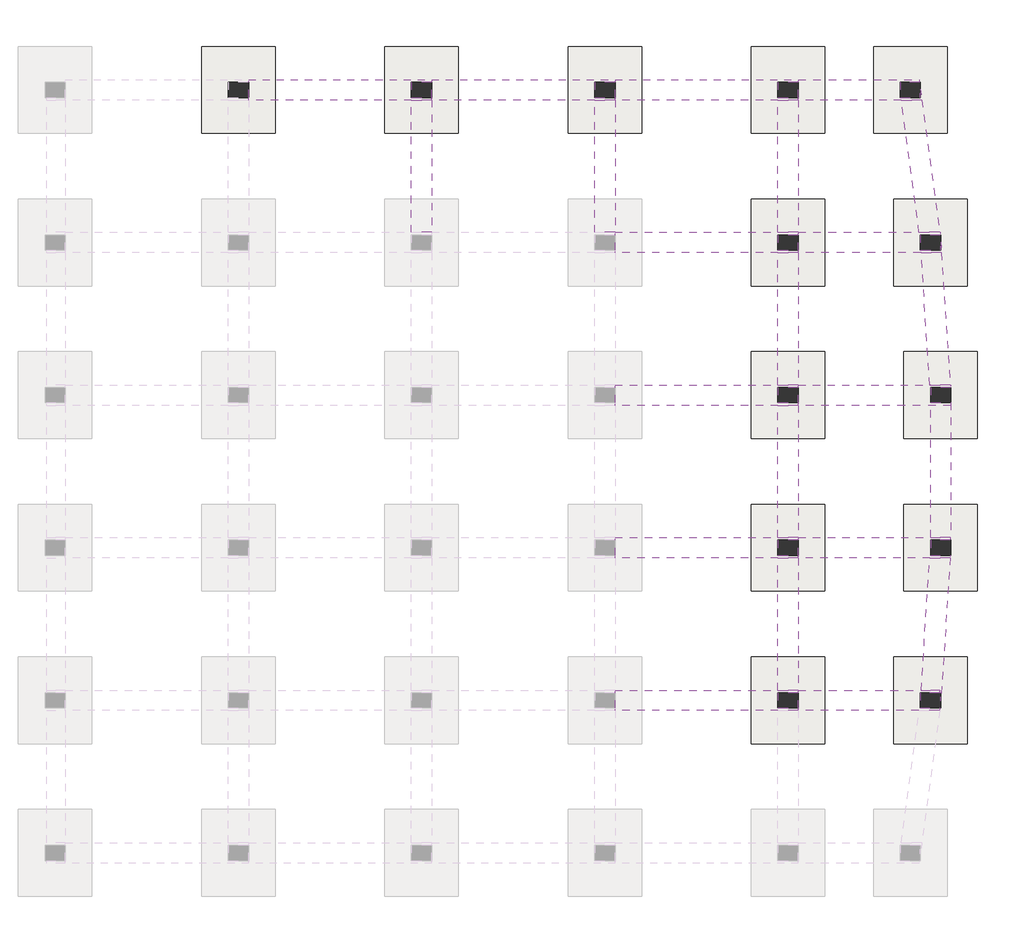
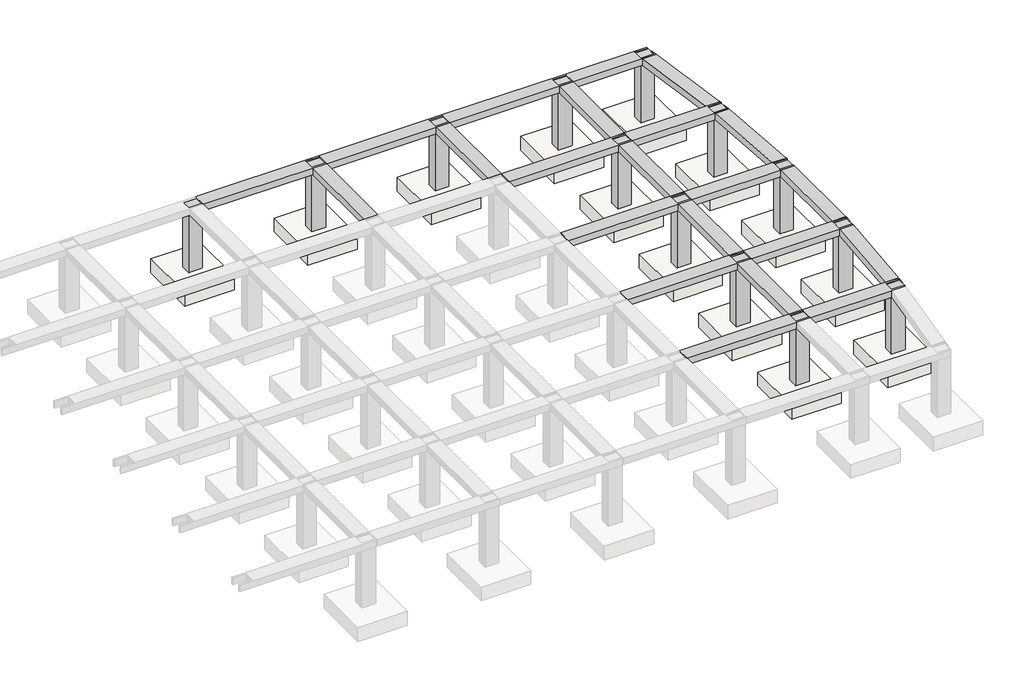
# One storey, part 3 of 3: 22 beams, 13 columns, 13 slabs.
"""IFC4 building model written with IfcOpenShell, lengths in millimetres."""

from ifc_helpers import new_model, si_unit, frame, origin, place, context, project, spatial, polyline, outline, extrude, faceted_brep, element, save

model = new_model("IFC4")

# Units and contexts
model_context = context("Model", 3, world=origin())
ifc_project = project(units=[si_unit("LENGTHUNIT", "METRE", prefix="MILLI")], contexts=[model_context])

# Site, building, storey
site = spatial("IfcSite", under=ifc_project)
building = spatial("IfcBuilding", under=site)
storey = spatial("IfcBuildingStorey", under=building, Elevation=-2999.978125)

# Beams
placement = place(None, origin())
element("IfcBeam", 1, ObjectType="Concrete-Rectangular Beam : 2' x2'", at=placement, inside=storey, context=model_context, shape_type="Brep", body=[
    faceted_brep([(-160.074232, 1680.7831222, 48.021875), (-160.074232, 1604.5831222, 48.021875), (-160.074232, 1147.3831222, 48.021875), (-160.074232, 1071.1831222, 48.021875), (4716.725768, 1071.1831222, 48.021875), (5326.325768, 1071.1831222, 48.021875), (5326.325768, 1147.3831222, 48.021875), (4716.725768, 1147.3831222, 48.021875), (4716.725768, 1604.5831222, 48.021875), (5326.325768, 1604.5831222, 48.021875), (5326.325768, 1680.7831222, 48.021875), (4716.725768, 1680.7831222, 48.021875), (-160.074232, 1071.1831222, -256.778125), (4716.725768, 1071.1831222, -256.778125), (5326.325768, 1071.1831222, -256.778125), (4716.725768, 1147.3831222, -256.778125), (5326.325768, 1147.3831222, -256.778125), (-160.074232, 1147.3831222, -256.778125), (-160.074232, 1604.5831222, -256.778125), (-160.074232, 1680.7831222, -256.778125), (4716.725768, 1680.7831222, -256.778125), (5326.325768, 1680.7831222, -256.778125), (5326.325768, 1604.5831222, -256.778125), (4716.725768, 1604.5831222, -256.778125)], [[[0, 1, 2, 3, 4, 5, 6, 7, 8, 9, 10, 11]], [[3, 12, 13, 14, 5, 4]], [[15, 16, 14, 13, 12, 17, 18, 19, 20, 21, 22, 23]], [[10, 21, 20, 19, 0, 11]], [[3, 2, 1, 0, 19, 18, 17, 12]], [[7, 6, 16, 15]], [[7, 15, 23, 8]], [[8, 23, 22, 9]], [[5, 14, 16, 6]], [[21, 10, 9, 22]]]),
])
element("IfcBeam", 2, ObjectType="Concrete-Rectangular Beam : 2' x2'", at=placement, inside=storey, context=model_context, shape_type="Brep", body=[
    faceted_brep([(9555.2251658, 1680.7831222, 48.021875), (9003.0522312, 1680.7831222, 48.021875), (5326.325768, 1680.7831222, 48.021875), (5326.325768, 1604.5831222, 48.021875), (5326.325768, 1147.3831222, 48.021875), (5326.325768, 1071.1831222, 48.021875), (8940.2370643, 1071.1831222, 48.021875), (9555.2251658, 1071.1831222, 48.021875), (9555.2251658, 1147.3831222, 48.021875), (8983.5457827, 1147.3831222, 48.021875), (8983.5457827, 1604.5831222, 48.021875), (9555.2251658, 1604.5831222, 48.021875), (9555.2251658, 1071.1831222, -256.778125), (5326.325768, 1071.1831222, -256.778125), (8940.2370643, 1071.1831222, -256.778125), (8983.5457827, 1147.3831222, -256.778125), (9555.2251658, 1147.3831222, -256.778125), (5326.325768, 1147.3831222, -256.778125), (5326.325768, 1604.5831222, -256.778125), (5326.325768, 1680.7831222, -256.778125), (9003.0522312, 1680.7831222, -256.778125), (9555.2251658, 1680.7831222, -256.778125), (9555.2251658, 1604.5831222, -256.778125), (8983.5457827, 1604.5831222, -256.778125)], [[[0, 1, 2, 3, 4, 5, 6, 7, 8, 9, 10, 11]], [[12, 7, 6, 5, 13, 14]], [[15, 16, 12, 14, 13, 17, 18, 19, 20, 21, 22, 23]], [[0, 21, 20, 19, 2, 1]], [[5, 4, 3, 2, 19, 18, 17, 13]], [[9, 8, 16, 15]], [[9, 15, 23, 10]], [[10, 23, 22, 11]], [[7, 12, 16, 8]], [[21, 0, 11, 22]]]),
])
element("IfcBeam", 3, ObjectType="Concrete-Rectangular Beam : 2' x2'", at=placement, inside=storey, context=model_context, shape_type="Brep", body=[
    faceted_brep([(-160.074232, 6252.7831222, 48.021875), (-160.074232, 6176.5831222, 48.021875), (-160.074232, 5719.3831222, 48.021875), (-160.074232, 5643.1831222, 48.021875), (4716.725768, 5643.1831222, 48.021875), (5326.325768, 5643.1831222, 48.021875), (5326.325768, 5719.3831222, 48.021875), (4716.725768, 5719.3831222, 48.021875), (4716.725768, 6176.5831222, 48.021875), (5326.325768, 6176.5831222, 48.021875), (5326.325768, 6252.7831222, 48.021875), (4716.725768, 6252.7831222, 48.021875), (-160.074232, 5643.1831222, -256.778125), (4716.725768, 5643.1831222, -256.778125), (5326.325768, 5643.1831222, -256.778125), (4716.725768, 5719.3831222, -256.778125), (5326.325768, 5719.3831222, -256.778125), (-160.074232, 5719.3831222, -256.778125), (-160.074232, 6176.5831222, -256.778125), (-160.074232, 6252.7831222, -256.778125), (4716.725768, 6252.7831222, -256.778125), (5326.325768, 6252.7831222, -256.778125), (5326.325768, 6176.5831222, -256.778125), (4716.725768, 6176.5831222, -256.778125)], [[[0, 1, 2, 3, 4, 5, 6, 7, 8, 9, 10, 11]], [[3, 12, 13, 14, 5, 4]], [[15, 16, 14, 13, 12, 17, 18, 19, 20, 21, 22, 23]], [[10, 21, 20, 19, 0, 11]], [[3, 2, 1, 0, 19, 18, 17, 12]], [[7, 6, 16, 15]], [[7, 15, 23, 8]], [[8, 23, 22, 9]], [[5, 14, 16, 6]], [[21, 10, 9, 22]]]),
])
element("IfcBeam", 4, ObjectType="Concrete-Rectangular Beam : 2' x2'", at=placement, inside=storey, context=model_context, shape_type="Brep", body=[
    faceted_brep([(9876.2389574, 6252.7831222, 48.021875), (9286.1454059, 6252.7831222, 48.021875), (5326.325768, 6252.7831222, 48.021875), (5326.325768, 6176.5831222, 48.021875), (5326.325768, 5719.3831222, 48.021875), (5326.325768, 5643.1831222, 48.021875), (9265.305238, 5643.1831222, 48.021875), (9876.2389574, 5643.1831222, 48.021875), (9876.2389574, 5719.3831222, 48.021875), (9286.1454059, 5719.3831222, 48.021875), (9286.1454059, 6176.5831222, 48.021875), (9876.2389574, 6176.5831222, 48.021875), (9876.2389574, 5643.1831222, -256.778125), (5326.325768, 5643.1831222, -256.778125), (9265.305238, 5643.1831222, -256.778125), (9286.1454059, 6176.5831222, -256.778125), (9286.1454059, 5719.3831222, -256.778125), (9876.2389574, 5719.3831222, -256.778125), (5326.325768, 5719.3831222, -256.778125), (5326.325768, 6176.5831222, -256.778125), (5326.325768, 6252.7831222, -256.778125), (9286.1454059, 6252.7831222, -256.778125), (9876.2389574, 6252.7831222, -256.778125), (9876.2389574, 6176.5831222, -256.778125), (9286.1454059, 5719.3831222, 0.0), (9286.1454059, 6176.5831222, 0.0)], [[[0, 1, 2, 3, 4, 5, 6, 7, 8, 9, 10, 11]], [[12, 7, 6, 5, 13, 14]], [[15, 16, 17, 12, 14, 13, 18, 19, 20, 21, 22, 23]], [[0, 22, 21, 20, 2, 1]], [[5, 4, 3, 2, 20, 19, 18, 13]], [[9, 8, 17, 16, 24]], [[10, 9, 24, 16, 15, 25]], [[10, 25, 15, 23, 11]], [[7, 12, 17, 8]], [[22, 0, 11, 23]]]),
])
element("IfcBeam", 5, ObjectType="Concrete-Rectangular Beam : 2' x2'", at=placement, inside=storey, context=model_context, shape_type="Brep", body=[
    faceted_brep([(-160.074232, 10824.7831222, 48.021875), (-160.074232, 10748.5831222, 48.021875), (-160.074232, 10291.3831222, 48.021875), (-160.074232, 10215.1831222, 48.021875), (4716.725768, 10215.1831222, 48.021875), (5326.325768, 10215.1831222, 48.021875), (5326.325768, 10291.3831222, 48.021875), (4716.725768, 10291.3831222, 48.021875), (4716.725768, 10748.5831222, 48.021875), (5326.325768, 10748.5831222, 48.021875), (5326.325768, 10824.7831222, 48.021875), (4716.725768, 10824.7831222, 48.021875), (-160.074232, 10215.1831222, -256.778125), (4716.725768, 10215.1831222, -256.778125), (5326.325768, 10215.1831222, -256.778125), (4716.725768, 10291.3831222, -256.778125), (5326.325768, 10291.3831222, -256.778125), (-160.074232, 10291.3831222, -256.778125), (-160.074232, 10748.5831222, -256.778125), (-160.074232, 10824.7831222, -256.778125), (4716.725768, 10824.7831222, -256.778125), (5326.325768, 10824.7831222, -256.778125), (5326.325768, 10748.5831222, -256.778125), (4716.725768, 10748.5831222, -256.778125)], [[[0, 1, 2, 3, 4, 5, 6, 7, 8, 9, 10, 11]], [[3, 12, 13, 14, 5, 4]], [[15, 16, 14, 13, 12, 17, 18, 19, 20, 21, 22, 23]], [[10, 21, 20, 19, 0, 11]], [[3, 2, 1, 0, 19, 18, 17, 12]], [[7, 6, 16, 15]], [[7, 15, 23, 8]], [[8, 23, 22, 9]], [[5, 14, 16, 6]], [[21, 10, 9, 22]]]),
])
element("IfcBeam", 6, ObjectType="Concrete-Rectangular Beam : 2' x2'", at=placement, inside=storey, context=model_context, shape_type="Brep", body=[
    faceted_brep([(9895.7454059, 10824.7831222, 48.021875), (9876.2389574, 10824.7831222, 48.021875), (9265.305238, 10824.7831222, 48.021875), (5326.325768, 10824.7831222, 48.021875), (5326.325768, 10748.5831222, 48.021875), (5326.325768, 10291.3831222, 48.021875), (5326.325768, 10215.1831222, 48.021875), (9895.7454059, 10215.1831222, 48.021875), (9895.7454059, 10291.3831222, 48.021875), (9286.1454059, 10291.3831222, 48.021875), (9286.1454059, 10748.5831222, 48.021875), (9895.7454059, 10748.5831222, 48.021875), (9895.7454059, 10215.1831222, -256.778125), (5326.325768, 10215.1831222, -256.778125), (9286.1454059, 10291.3831222, -256.778125), (9895.7454059, 10291.3831222, -256.778125), (5326.325768, 10291.3831222, -256.778125), (5326.325768, 10748.5831222, -256.778125), (5326.325768, 10824.7831222, -256.778125), (9265.305238, 10824.7831222, -256.778125), (9876.2389574, 10824.7831222, -256.778125), (9895.7454059, 10824.7831222, -256.778125), (9895.7454059, 10748.5831222, -256.778125), (9286.1454059, 10748.5831222, -256.778125), (9895.7454059, 10291.3831222, 0.0), (9286.1454059, 10291.3831222, 0.0), (9286.1454059, 10748.5831222, 0.0), (9895.7454059, 10748.5831222, 0.0)], [[[0, 1, 2, 3, 4, 5, 6, 7, 8, 9, 10, 11]], [[12, 7, 6, 13]], [[14, 15, 12, 13, 16, 17, 18, 19, 20, 21, 22, 23]], [[0, 21, 20, 19, 18, 3, 2, 1]], [[6, 5, 4, 3, 18, 17, 16, 13]], [[9, 8, 24, 15, 14, 25]], [[9, 25, 14, 23, 26, 10]], [[10, 26, 23, 22, 27, 11]], [[7, 12, 15, 24, 8]], [[21, 0, 11, 27, 22]]]),
])
element("IfcBeam", 7, ObjectType="Concrete-Rectangular Beam : 2' x2'", at=placement, inside=storey, context=model_context, shape_type="Brep", body=[
    faceted_brep([(-160.074232, 15396.7831222, 48.021875), (-160.074232, 15320.5831222, 48.021875), (-160.074232, 14863.3831222, 48.021875), (-160.074232, 14787.1831222, 48.021875), (4716.725768, 14787.1831222, 48.021875), (5326.325768, 14787.1831222, 48.021875), (5326.325768, 14863.3831222, 48.021875), (4716.725768, 14863.3831222, 48.021875), (4716.725768, 15320.5831222, 48.021875), (5326.325768, 15320.5831222, 48.021875), (5326.325768, 15396.7831222, 48.021875), (4716.725768, 15396.7831222, 48.021875), (-160.074232, 14787.1831222, -256.778125), (4716.725768, 14787.1831222, -256.778125), (5326.325768, 14787.1831222, -256.778125), (4716.725768, 14863.3831222, -256.778125), (5326.325768, 14863.3831222, -256.778125), (-160.074232, 14863.3831222, -256.778125), (-160.074232, 15320.5831222, -256.778125), (-160.074232, 15396.7831222, -256.778125), (4716.725768, 15396.7831222, -256.778125), (5326.325768, 15396.7831222, -256.778125), (5326.325768, 15320.5831222, -256.778125), (4716.725768, 15320.5831222, -256.778125)], [[[0, 1, 2, 3, 4, 5, 6, 7, 8, 9, 10, 11]], [[3, 12, 13, 14, 5, 4]], [[15, 16, 14, 13, 12, 17, 18, 19, 20, 21, 22, 23]], [[10, 21, 20, 19, 0, 11]], [[3, 2, 1, 0, 19, 18, 17, 12]], [[7, 6, 16, 15]], [[7, 15, 23, 8]], [[8, 23, 22, 9]], [[5, 14, 16, 6]], [[21, 10, 9, 22]]]),
])
element("IfcBeam", 8, ObjectType="Concrete-Rectangular Beam : 2' x2'", at=placement, inside=storey, context=model_context, shape_type="Brep", body=[
    faceted_brep([(9573.6393342, 15396.7831222, 48.021875), (9555.2251658, 15396.7831222, 48.021875), (8940.2370643, 15396.7831222, 48.021875), (5326.325768, 15396.7831222, 48.021875), (5326.325768, 15320.5831222, 48.021875), (5326.325768, 14863.3831222, 48.021875), (5326.325768, 14787.1831222, 48.021875), (9003.0522312, 14787.1831222, 48.021875), (9613.9859506, 14787.1831222, 48.021875), (9593.1457827, 15102.0587543, 48.021875), (9593.1457827, 14863.3831222, 48.021875), (8983.5457827, 14863.3831222, 48.021875), (8983.5457827, 15320.5831222, 48.021875), (9578.6826612, 15320.5831222, 48.021875), (9613.9859506, 14787.1831222, -256.778125), (5326.325768, 14787.1831222, -256.778125), (9003.0522312, 14787.1831222, -256.778125), (8983.5457827, 14863.3831222, -256.778125), (9593.1457827, 14863.3831222, -256.778125), (9593.1457827, 15102.0587543, -256.778125), (5326.325768, 14863.3831222, -256.778125), (5326.325768, 15320.5831222, -256.778125), (5326.325768, 15396.7831222, -256.778125), (8940.2370643, 15396.7831222, -256.778125), (9555.2251658, 15396.7831222, -256.778125), (9573.6393342, 15396.7831222, -256.778125), (9578.6826612, 15320.5831222, -256.778125), (8983.5457827, 15320.5831222, -256.778125)], [[[0, 1, 2, 3, 4, 5, 6, 7, 8, 9, 10, 11, 12, 13]], [[14, 8, 7, 6, 15, 16]], [[17, 18, 19, 14, 16, 15, 20, 21, 22, 23, 24, 25, 26, 27]], [[0, 25, 24, 23, 22, 3, 2, 1]], [[6, 5, 4, 3, 22, 21, 20, 15]], [[11, 10, 18, 17]], [[11, 17, 27, 12]], [[12, 27, 26, 13]], [[8, 14, 19, 9]], [[18, 10, 9, 19]], [[25, 0, 13, 26]]]),
])
element("IfcBeam", 9, ObjectType="Concrete-Rectangular Beam : 2' x2'", at=placement, inside=storey, context=model_context, shape_type="Brep", body=[
    faceted_brep([(-11132.874232, 19968.7831222, 48.021875), (-11132.874232, 19892.5831222, 48.021875), (-11132.874232, 19435.3831222, 48.021875), (-11132.874232, 19359.1831222, 48.021875), (-6256.074232, 19359.1831222, 48.021875), (-5646.474232, 19359.1831222, 48.021875), (-5646.474232, 19435.3831222, 48.021875), (-6256.074232, 19435.3831222, 48.021875), (-6256.074232, 19892.5831222, 48.021875), (-5646.474232, 19892.5831222, 48.021875), (-5646.474232, 19968.7831222, 48.021875), (-11132.874232, 19359.1831222, -256.778125), (-6256.074232, 19359.1831222, -256.778125), (-5646.474232, 19359.1831222, -256.778125), (-6256.074232, 19435.3831222, -256.778125), (-5646.474232, 19435.3831222, -256.778125), (-11132.874232, 19435.3831222, -256.778125), (-11132.874232, 19892.5831222, -256.778125), (-11132.874232, 19968.7831222, -256.778125), (-5646.474232, 19968.7831222, -256.778125), (-5646.474232, 19892.5831222, -256.778125), (-6256.074232, 19892.5831222, -256.778125)], [[[0, 1, 2, 3, 4, 5, 6, 7, 8, 9, 10]], [[3, 11, 12, 13, 5, 4]], [[14, 15, 13, 12, 11, 16, 17, 18, 19, 20, 21]], [[10, 19, 18, 0]], [[3, 2, 1, 0, 18, 17, 16, 11]], [[7, 6, 15, 14]], [[7, 14, 21, 8]], [[8, 21, 20, 9]], [[5, 13, 15, 6]], [[19, 10, 9, 20]]]),
])
element("IfcBeam", 10, ObjectType="Concrete-Rectangular Beam : 2' x2'", at=placement, inside=storey, context=model_context, shape_type="Brep", body=[
    faceted_brep([(-160.074232, 19968.7831222, 48.021875), (-5646.474232, 19968.7831222, 48.021875), (-5646.474232, 19892.5831222, 48.021875), (-5646.474232, 19435.3831222, 48.021875), (-5646.474232, 19359.1831222, 48.021875), (-769.674232, 19359.1831222, 48.021875), (-160.074232, 19359.1831222, 48.021875), (-160.074232, 19435.3831222, 48.021875), (-769.674232, 19435.3831222, 48.021875), (-769.674232, 19892.5831222, 48.021875), (-160.074232, 19892.5831222, 48.021875), (-160.074232, 19359.1831222, -256.778125), (-5646.474232, 19359.1831222, -256.778125), (-769.674232, 19359.1831222, -256.778125), (-769.674232, 19435.3831222, -256.778125), (-160.074232, 19435.3831222, -256.778125), (-5646.474232, 19435.3831222, -256.778125), (-5646.474232, 19892.5831222, -256.778125), (-5646.474232, 19968.7831222, -256.778125), (-160.074232, 19968.7831222, -256.778125), (-160.074232, 19892.5831222, -256.778125), (-769.674232, 19892.5831222, -256.778125)], [[[0, 1, 2, 3, 4, 5, 6, 7, 8, 9, 10]], [[11, 6, 5, 4, 12, 13]], [[14, 15, 11, 13, 12, 16, 17, 18, 19, 20, 21]], [[0, 19, 18, 1]], [[4, 3, 2, 1, 18, 17, 16, 12]], [[8, 7, 15, 14]], [[8, 14, 21, 9]], [[9, 21, 20, 10]], [[6, 11, 15, 7]], [[19, 0, 10, 20]]]),
])
element("IfcBeam", 11, ObjectType="Concrete-Rectangular Beam : 2' x2'", at=placement, inside=storey, context=model_context, shape_type="Brep", body=[
    faceted_brep([(-160.074232, 19968.7831222, 48.021875), (-160.074232, 19892.5831222, 48.021875), (-160.074232, 19435.3831222, 48.021875), (-160.074232, 19359.1831222, 48.021875), (4716.725768, 19359.1831222, 48.021875), (5326.325768, 19359.1831222, 48.021875), (5326.325768, 19435.3831222, 48.021875), (4716.725768, 19435.3831222, 48.021875), (4716.725768, 19892.5831222, 48.021875), (5326.325768, 19892.5831222, 48.021875), (5326.325768, 19968.7831222, 48.021875), (-160.074232, 19359.1831222, -256.778125), (4716.725768, 19359.1831222, -256.778125), (5326.325768, 19359.1831222, -256.778125), (4716.725768, 19435.3831222, -256.778125), (5326.325768, 19435.3831222, -256.778125), (-160.074232, 19435.3831222, -256.778125), (-160.074232, 19892.5831222, -256.778125), (-160.074232, 19968.7831222, -256.778125), (5326.325768, 19968.7831222, -256.778125), (5326.325768, 19892.5831222, -256.778125), (4716.725768, 19892.5831222, -256.778125)], [[[0, 1, 2, 3, 4, 5, 6, 7, 8, 9, 10]], [[3, 11, 12, 13, 5, 4]], [[14, 15, 13, 12, 11, 16, 17, 18, 19, 20, 21]], [[10, 19, 18, 0]], [[3, 2, 1, 0, 18, 17, 16, 11]], [[7, 6, 15, 14]], [[7, 14, 21, 8]], [[8, 21, 20, 9]], [[5, 13, 15, 6]], [[19, 10, 9, 20]]]),
])
element("IfcBeam", 12, ObjectType="Concrete-Rectangular Beam : 2' x2'", at=placement, inside=storey, context=model_context, shape_type="Brep", body=[
    faceted_brep([(5326.325768, 19968.7831222, 48.021875), (5326.325768, 19892.5831222, 48.021875), (5326.325768, 19435.3831222, 48.021875), (5326.325768, 19359.1831222, 48.021875), (8412.2463849, 19359.1831222, 48.021875), (9027.2344863, 19359.1831222, 48.021875), (8983.925768, 19684.2011052, 48.021875), (8983.925768, 19435.3831222, 48.021875), (8374.325768, 19435.3831222, 48.021875), (8374.325768, 19892.5831222, 48.021875), (8956.158818, 19892.5831222, 48.021875), (8946.005151, 19968.7831222, 48.021875), (5326.325768, 19359.1831222, -256.778125), (8412.2463849, 19359.1831222, -256.778125), (9027.2344863, 19359.1831222, -256.778125), (8374.325768, 19435.3831222, -256.778125), (8983.925768, 19435.3831222, -256.778125), (8983.925768, 19684.2011052, -256.778125), (5326.325768, 19435.3831222, -256.778125), (5326.325768, 19892.5831222, -256.778125), (5326.325768, 19968.7831222, -256.778125), (8946.005151, 19968.7831222, -256.778125), (8956.158818, 19892.5831222, -256.778125), (8374.325768, 19892.5831222, -256.778125)], [[[0, 1, 2, 3, 4, 5, 6, 7, 8, 9, 10, 11]], [[3, 12, 13, 14, 5, 4]], [[15, 16, 17, 14, 13, 12, 18, 19, 20, 21, 22, 23]], [[11, 21, 20, 0]], [[3, 2, 1, 0, 20, 19, 18, 12]], [[8, 7, 16, 15]], [[8, 15, 23, 9]], [[9, 23, 22, 10]], [[5, 14, 17, 6]], [[16, 7, 6, 17]], [[21, 11, 10, 22]]]),
])
element("IfcBeam", 13, ObjectType="Concrete-Rectangular Beam : 2' x2'", at=placement, inside=storey, context=model_context, shape_type="SweptSolid", body=[
    extrude(outline(polyline([(-5646.474232, 15396.7831222), (-6256.074232, 15396.7831222), (-6256.074232, 19359.1831222), (-5646.474232, 19359.1831222), (-5646.474232, 15396.7831222)])), frame((0.0, 0.0, -256.778125), z_axis=(0.0, 0.0, 1.0), x_axis=(1.0, 0.0, 0.0)), (0.0, 0.0, 1.0), 304.8),
])
element("IfcBeam", 14, ObjectType="Concrete-Rectangular Beam : 2' x2'", at=placement, inside=storey, context=model_context, shape_type="SweptSolid", body=[
    extrude(outline(polyline([(-160.074232, 15396.7831222), (-769.674232, 15396.7831222), (-769.674232, 19359.1831222), (-160.074232, 19359.1831222), (-160.074232, 15396.7831222)])), frame((0.0, 0.0, -256.778125), z_axis=(0.0, 0.0, 1.0), x_axis=(1.0, 0.0, 0.0)), (0.0, 0.0, 1.0), 304.8),
])
element("IfcBeam", 15, ObjectType="Concrete-Rectangular Beam : 2' x2'", at=placement, inside=storey, context=model_context, shape_type="SweptSolid", body=[
    extrude(outline(polyline([(5326.325768, 1680.7831222), (4716.725768, 1680.7831222), (4716.725768, 5643.1831222), (5326.325768, 5643.1831222), (5326.325768, 1680.7831222)])), frame((0.0, 0.0, -256.778125), z_axis=(0.0, 0.0, 1.0), x_axis=(1.0, 0.0, 0.0)), (0.0, 0.0, 1.0), 304.8),
])
element("IfcBeam", 16, ObjectType="Concrete-Rectangular Beam : 2' x2'", at=placement, inside=storey, context=model_context, shape_type="SweptSolid", body=[
    extrude(outline(polyline([(4716.725768, 10215.1831222), (5326.325768, 10215.1831222), (5326.325768, 6252.7831222), (4716.725768, 6252.7831222), (4716.725768, 10215.1831222)])), frame((0.0, 0.0, -256.778125), z_axis=(0.0, 0.0, 1.0), x_axis=(1.0, 0.0, 0.0)), (0.0, 0.0, 1.0), 304.8),
])
element("IfcBeam", 17, ObjectType="Concrete-Rectangular Beam : 2' x2'", at=placement, inside=storey, context=model_context, shape_type="SweptSolid", body=[
    extrude(outline(polyline([(4716.725768, 14787.1831222), (5326.325768, 14787.1831222), (5326.325768, 10824.7831222), (4716.725768, 10824.7831222), (4716.725768, 14787.1831222)])), frame((0.0, 0.0, -256.778125), z_axis=(0.0, 0.0, 1.0), x_axis=(1.0, 0.0, 0.0)), (0.0, 0.0, 1.0), 304.8),
])
element("IfcBeam", 18, ObjectType="Concrete-Rectangular Beam : 2' x2'", at=placement, inside=storey, context=model_context, shape_type="SweptSolid", body=[
    extrude(outline(polyline([(5326.325768, 15396.7831222), (4716.725768, 15396.7831222), (4716.725768, 19359.1831222), (5326.325768, 19359.1831222), (5326.325768, 15396.7831222)])), frame((0.0, 0.0, -256.778125), z_axis=(0.0, 0.0, 1.0), x_axis=(1.0, 0.0, 0.0)), (0.0, 0.0, 1.0), 304.8),
])
element("IfcBeam", 19, ObjectType="Concrete-Rectangular Beam : 2' x2'", at=placement, inside=storey, context=model_context, shape_type="Brep", body=[
    faceted_brep([(9916.5855738, 6252.7831222, 48.021875), (9895.7454059, 6252.7831222, 48.021875), (9876.2389574, 6252.7831222, 48.021875), (9876.2389574, 6176.5831222, 48.021875), (9895.7454059, 6176.5831222, 48.021875), (9895.7454059, 5937.9074901, 48.021875), (9916.5855738, 6252.7831222, -256.778125), (9895.7454059, 5937.9074901, -256.778125), (9895.7454059, 6176.5831222, -256.778125), (9876.2389574, 6176.5831222, -256.778125), (9876.2389574, 6252.7831222, -256.778125), (9895.7454059, 6252.7831222, -256.778125)], [[[0, 1, 2, 3, 4, 5]], [[6, 0, 5, 7]], [[6, 7, 8, 9, 10, 11]], [[0, 6, 11, 10, 2, 1]], [[8, 7, 5, 4]], [[8, 4, 3, 9]], [[10, 9, 3, 2]]]),
    faceted_brep([(9003.0522312, 1680.7831222, -256.778125), (9003.0522312, 1680.7831222, 48.021875), (9265.305238, 5643.1831222, 48.021875), (9265.305238, 5643.1831222, -256.778125), (9593.1457827, 1604.5831222, -256.778125), (9593.1457827, 1365.9074901, -256.778125), (9593.1457827, 1365.9074901, 48.021875), (9593.1457827, 1604.5831222, 48.021875), (9555.2251658, 1604.5831222, -256.778125), (9555.2251658, 1604.5831222, 48.021875), (9881.2822845, 5719.3831222, -256.778125), (9876.2389574, 5719.3831222, -256.778125), (9876.2389574, 5719.3831222, 48.021875), (9881.2822845, 5719.3831222, 48.021875), (9021.4663996, 1680.7831222, -256.778125), (9555.2251658, 1680.7831222, -256.778125), (9555.2251658, 1680.7831222, 48.021875), (9021.4663996, 1680.7831222, 48.021875), (9876.2389574, 5643.1831222, 48.021875), (9876.2389574, 5643.1831222, -256.778125)], [[[0, 1, 2, 3]], [[4, 5, 6, 7]], [[8, 4, 7, 9]], [[10, 11, 12, 13]], [[1, 0, 14, 15, 16, 17]], [[2, 18, 19, 3]], [[11, 10, 19]], [[19, 18, 12, 11]], [[18, 2, 1, 17, 16, 9, 7, 6]], [[5, 4, 8, 15, 14, 0, 3, 19]], [[16, 15, 8, 9]], [[12, 18, 13]], [[10, 13, 18, 6, 5, 19]]]),
    faceted_brep([(9555.2251658, 1071.1831222, -256.778125), (9565.3788327, 1147.3831222, -256.778125), (9565.3788327, 1147.3831222, 48.021875), (9555.2251658, 1071.1831222, 48.021875), (9555.2251658, 1147.3831222, -256.778125), (9555.2251658, 1147.3831222, 48.021875)], [[[0, 1, 2, 3]], [[1, 4, 5, 2]], [[1, 0, 4]], [[0, 3, 5, 4]], [[3, 2, 5]]]),
])
element("IfcBeam", 20, ObjectType="Concrete-Rectangular Beam : 2' x2'", at=placement, inside=storey, context=model_context, shape_type="Brep", body=[
    faceted_brep([(9895.7454059, 10824.7831222, 48.021875), (9876.2389574, 10824.7831222, 48.021875), (9286.1454059, 10824.7831222, 48.021875), (9286.1454059, 10748.5831222, 48.021875), (9895.7454059, 10748.5831222, 48.021875), (9895.7454059, 10824.7831222, -256.778125), (9895.7454059, 10748.5831222, -256.778125), (9286.1454059, 10824.7831222, -256.778125), (9876.2389574, 10824.7831222, -256.778125), (9286.1454059, 10748.5831222, -256.778125)], [[[0, 1, 2, 3, 4]], [[5, 0, 4, 6]], [[7, 8, 5, 6, 9]], [[2, 7, 9, 3]], [[2, 1, 0, 5, 8, 7]], [[4, 3, 9, 6]]]),
    faceted_brep([(9895.7454059, 10291.3831222, -256.778125), (9286.1454059, 10291.3831222, -256.778125), (9286.1454059, 10291.3831222, 48.021875), (9895.7454059, 10291.3831222, 48.021875), (9286.1454059, 6252.7831222, 48.021875), (9286.1454059, 6252.7831222, -256.778125), (9876.2389574, 6252.7831222, -256.778125), (9895.7454059, 6252.7831222, -256.778125), (9895.7454059, 6252.7831222, 48.021875), (9876.2389574, 6252.7831222, 48.021875)], [[[0, 1, 2, 3]], [[4, 5, 6, 7, 8, 9]], [[1, 0, 7, 6, 5]], [[4, 9, 8, 3, 2]], [[0, 3, 8, 7]], [[2, 1, 5, 4]]]),
])
element("IfcBeam", 21, ObjectType="Concrete-Rectangular Beam : 2' x2'", at=placement, inside=storey, context=model_context, shape_type="Brep", body=[
    faceted_brep([(9613.9859506, 14787.1831222, 48.021875), (9003.0522312, 14787.1831222, 48.021875), (9265.305238, 10824.7831222, 48.021875), (9286.1454059, 10824.7831222, 48.021875), (9876.2389574, 10824.7831222, 48.021875), (9613.9859506, 14787.1831222, -256.778125), (9876.2389574, 10824.7831222, -256.778125), (9003.0522312, 14787.1831222, -256.778125), (9286.1454059, 10824.7831222, -256.778125), (9265.305238, 10824.7831222, -256.778125)], [[[0, 1, 2, 3, 4]], [[5, 0, 4, 6]], [[7, 5, 6, 8, 9]], [[1, 7, 9, 2]], [[1, 0, 5, 7]], [[4, 3, 2, 9, 8, 6]]]),
])
element("IfcBeam", 22, ObjectType="Concrete-Rectangular Beam : 2' x2'", at=placement, inside=storey, context=model_context, shape_type="SweptSolid", body=[
    extrude(outline(polyline([(8412.2463849, 19359.1831222), (9027.2344863, 19359.1831222), (9555.2251658, 15396.7831222), (8940.2370643, 15396.7831222), (8412.2463849, 19359.1831222)])), frame((0.0, 0.0, -256.778125), z_axis=(0.0, 0.0, 1.0), x_axis=(1.0, 0.0, 0.0)), (0.0, 0.0, 1.0), 304.8),
])

# Columns
element("IfcColumn", 23, ObjectType="Concrete-Rectangular-Column : 12 x 18", at=placement, inside=storey, context=model_context, shape_type="SweptSolid", body=[
    extrude(outline(polyline([(5326.325768, 1604.5831222), (5326.325768, 1147.3831222), (4716.725768, 1147.3831222), (4716.725768, 1604.5831222), (5326.325768, 1604.5831222)])), frame((0.0, 0.0, -2999.978125), z_axis=(0.0, 0.0, 1.0), x_axis=(1.0, 0.0, 0.0)), (0.0, 0.0, 1.0), 2999.978125),
])
element("IfcColumn", 24, ObjectType="Concrete-Rectangular-Column : 12 x 18", at=placement, inside=storey, context=model_context, shape_type="SweptSolid", body=[
    extrude(outline(polyline([(9593.1457827, 1604.5831222), (9593.1457827, 1147.3831222), (8983.5457827, 1147.3831222), (8983.5457827, 1604.5831222), (9593.1457827, 1604.5831222)])), frame((0.0, 0.0, -2999.978125), z_axis=(0.0, 0.0, 1.0), x_axis=(1.0, 0.0, 0.0)), (0.0, 0.0, 1.0), 2999.978125),
])
element("IfcColumn", 25, ObjectType="Concrete-Rectangular-Column : 12 x 18", at=placement, inside=storey, context=model_context, shape_type="SweptSolid", body=[
    extrude(outline(polyline([(5326.325768, 6176.5831222), (5326.325768, 5719.3831222), (4716.725768, 5719.3831222), (4716.725768, 6176.5831222), (5326.325768, 6176.5831222)])), frame((0.0, 0.0, -2999.978125), z_axis=(0.0, 0.0, 1.0), x_axis=(1.0, 0.0, 0.0)), (0.0, 0.0, 1.0), 2999.978125),
])
element("IfcColumn", 26, ObjectType="Concrete-Rectangular-Column : 12 x 18", at=placement, inside=storey, context=model_context, shape_type="Brep", body=[
    faceted_brep([(9895.7454059, 6176.5831222, -2999.978125), (9895.7454059, 5719.3831222, -2999.978125), (9286.1454059, 5719.3831222, -2999.978125), (9286.1454059, 6176.5831222, -2999.978125), (9895.7454059, 6176.5831222, 0.0), (9895.7454059, 5719.3831222, 0.0), (9286.1454059, 5719.3831222, 0.0), (9286.1454059, 5719.3831222, -256.778125), (9286.1454059, 6176.5831222, 0.0), (9286.1454059, 6176.5831222, -256.778125)], [[[0, 1, 2, 3]], [[4, 5, 1, 0]], [[5, 6, 7, 2, 1]], [[6, 8, 9, 3, 2, 7]], [[8, 4, 0, 3, 9]], [[4, 8, 6, 5]]]),
])
element("IfcColumn", 27, ObjectType="Concrete-Rectangular-Column : 12 x 18", at=placement, inside=storey, context=model_context, shape_type="SweptSolid", body=[
    extrude(outline(polyline([(5326.325768, 10748.5831222), (5326.325768, 10291.3831222), (4716.725768, 10291.3831222), (4716.725768, 10748.5831222), (5326.325768, 10748.5831222)])), frame((0.0, 0.0, -2999.978125), z_axis=(0.0, 0.0, 1.0), x_axis=(1.0, 0.0, 0.0)), (0.0, 0.0, 1.0), 2999.978125),
])
element("IfcColumn", 28, ObjectType="Concrete-Rectangular-Column : 12 x 18", at=placement, inside=storey, context=model_context, shape_type="Brep", body=[
    faceted_brep([(9895.7454059, 10748.5831222, -2999.978125), (9895.7454059, 10291.3831222, -2999.978125), (9286.1454059, 10291.3831222, -2999.978125), (9286.1454059, 10748.5831222, -2999.978125), (9895.7454059, 10748.5831222, 0.0), (9895.7454059, 10291.3831222, 0.0), (9895.7454059, 10291.3831222, -256.778125), (9895.7454059, 10748.5831222, -256.778125), (9286.1454059, 10291.3831222, 0.0), (9286.1454059, 10291.3831222, -256.778125), (9286.1454059, 10748.5831222, 0.0), (9286.1454059, 10748.5831222, -256.778125)], [[[0, 1, 2, 3]], [[4, 5, 6, 1, 0, 7]], [[5, 8, 9, 2, 1, 6]], [[8, 10, 11, 3, 2, 9]], [[10, 4, 7, 0, 3, 11]], [[4, 10, 8, 5]]]),
])
element("IfcColumn", 29, ObjectType="Concrete-Rectangular-Column : 12 x 18", at=placement, inside=storey, context=model_context, shape_type="SweptSolid", body=[
    extrude(outline(polyline([(5326.325768, 15320.5831222), (5326.325768, 14863.3831222), (4716.725768, 14863.3831222), (4716.725768, 15320.5831222), (5326.325768, 15320.5831222)])), frame((0.0, 0.0, -2999.978125), z_axis=(0.0, 0.0, 1.0), x_axis=(1.0, 0.0, 0.0)), (0.0, 0.0, 1.0), 2999.978125),
])
element("IfcColumn", 30, ObjectType="Concrete-Rectangular-Column : 12 x 18", at=placement, inside=storey, context=model_context, shape_type="SweptSolid", body=[
    extrude(outline(polyline([(9593.1457827, 15320.5831222), (9593.1457827, 14863.3831222), (8983.5457827, 14863.3831222), (8983.5457827, 15320.5831222), (9593.1457827, 15320.5831222)])), frame((0.0, 0.0, -2999.978125), z_axis=(0.0, 0.0, 1.0), x_axis=(1.0, 0.0, 0.0)), (0.0, 0.0, 1.0), 2999.978125),
])
element("IfcColumn", 31, ObjectType="Concrete-Rectangular-Column : 12 x 18", at=placement, inside=storey, context=model_context, shape_type="SweptSolid", body=[
    extrude(outline(polyline([(-11132.874232, 19892.5831222), (-11132.874232, 19435.3831222), (-11742.474232, 19435.3831222), (-11742.474232, 19892.5831222), (-11132.874232, 19892.5831222)])), frame((0.0, 0.0, -2999.978125), z_axis=(0.0, 0.0, 1.0), x_axis=(1.0, 0.0, 0.0)), (0.0, 0.0, 1.0), 2999.978125),
])
element("IfcColumn", 32, ObjectType="Concrete-Rectangular-Column : 12 x 18", at=placement, inside=storey, context=model_context, shape_type="SweptSolid", body=[
    extrude(outline(polyline([(-5646.474232, 19892.5831222), (-5646.474232, 19435.3831222), (-6256.074232, 19435.3831222), (-6256.074232, 19892.5831222), (-5646.474232, 19892.5831222)])), frame((0.0, 0.0, -2999.978125), z_axis=(0.0, 0.0, 1.0), x_axis=(1.0, 0.0, 0.0)), (0.0, 0.0, 1.0), 2999.978125),
])
element("IfcColumn", 33, ObjectType="Concrete-Rectangular-Column : 12 x 18", at=placement, inside=storey, context=model_context, shape_type="SweptSolid", body=[
    extrude(outline(polyline([(-160.074232, 19892.5831222), (-160.074232, 19435.3831222), (-769.674232, 19435.3831222), (-769.674232, 19892.5831222), (-160.074232, 19892.5831222)])), frame((0.0, 0.0, -2999.978125), z_axis=(0.0, 0.0, 1.0), x_axis=(1.0, 0.0, 0.0)), (0.0, 0.0, 1.0), 2999.978125),
])
element("IfcColumn", 34, ObjectType="Concrete-Rectangular-Column : 12 x 18", at=placement, inside=storey, context=model_context, shape_type="SweptSolid", body=[
    extrude(outline(polyline([(5326.325768, 19892.5831222), (5326.325768, 19435.3831222), (4716.725768, 19435.3831222), (4716.725768, 19892.5831222), (5326.325768, 19892.5831222)])), frame((0.0, 0.0, -2999.978125), z_axis=(0.0, 0.0, 1.0), x_axis=(1.0, 0.0, 0.0)), (0.0, 0.0, 1.0), 2999.978125),
])
element("IfcColumn", 35, ObjectType="Concrete-Rectangular-Column : 12 x 18", at=placement, inside=storey, context=model_context, shape_type="SweptSolid", body=[
    extrude(outline(polyline([(8983.925768, 19892.5831222), (8983.925768, 19435.3831222), (8374.325768, 19435.3831222), (8374.325768, 19892.5831222), (8983.925768, 19892.5831222)])), frame((0.0, 0.0, -2999.978125), z_axis=(0.0, 0.0, 1.0), x_axis=(1.0, 0.0, 0.0)), (0.0, 0.0, 1.0), 2999.978125),
])

# Slabs
element("IfcSlab", 36, ObjectType="Footing-Rectangular : 650 X 2200X2600", at=placement, inside=storey, context=model_context, shape_type="SweptSolid", body=[
    extrude(outline(polyline([(6121.5144398, 2675.9967941), (6121.5144398, 75.9694503), (3921.5370961, 75.9694503), (3921.5370961, 2675.9967941), (6121.5144398, 2675.9967941)])), frame((0.0, 0.0, -3649.9601562), z_axis=(0.0, 0.0, 1.0), x_axis=(1.0, 0.0, 0.0)), (0.0, 0.0, 1.0), 649.9820313),
])
element("IfcSlab", 37, ObjectType="Footing-Rectangular : 650 X 2200X2600", at=placement, inside=storey, context=model_context, shape_type="SweptSolid", body=[
    extrude(outline(polyline([(10388.3344546, 2675.9967941), (10388.3344546, 75.9694503), (8188.3571108, 75.9694503), (8188.3571108, 2675.9967941), (10388.3344546, 2675.9967941)])), frame((0.0, 0.0, -3649.9601562), z_axis=(0.0, 0.0, 1.0), x_axis=(1.0, 0.0, 0.0)), (0.0, 0.0, 1.0), 649.9820313),
])
element("IfcSlab", 38, ObjectType="Footing-Rectangular : 650 X 2200X2600", at=placement, inside=storey, context=model_context, shape_type="SweptSolid", body=[
    extrude(outline(polyline([(6121.5144398, 7247.9967941), (6121.5144398, 4647.9694503), (3921.5370961, 4647.9694503), (3921.5370961, 7247.9967941), (6121.5144398, 7247.9967941)])), frame((0.0, 0.0, -3649.9601562), z_axis=(0.0, 0.0, 1.0), x_axis=(1.0, 0.0, 0.0)), (0.0, 0.0, 1.0), 649.9820313),
])
element("IfcSlab", 39, ObjectType="Footing-Rectangular : 650 X 2200X2600", at=placement, inside=storey, context=model_context, shape_type="SweptSolid", body=[
    extrude(outline(polyline([(10690.9340778, 7247.9967941), (10690.9340778, 4647.9694503), (8490.9567341, 4647.9694503), (8490.9567341, 7247.9967941), (10690.9340778, 7247.9967941)])), frame((0.0, 0.0, -3649.9601562), z_axis=(0.0, 0.0, 1.0), x_axis=(1.0, 0.0, 0.0)), (0.0, 0.0, 1.0), 649.9820313),
])
element("IfcSlab", 40, ObjectType="Footing-Rectangular : 650 X 2200X2600", at=placement, inside=storey, context=model_context, shape_type="SweptSolid", body=[
    extrude(outline(polyline([(6121.5144398, 11819.9967941), (6121.5144398, 9219.9694503), (3921.5370961, 9219.9694503), (3921.5370961, 11819.9967941), (6121.5144398, 11819.9967941)])), frame((0.0, 0.0, -3649.9601562), z_axis=(0.0, 0.0, 1.0), x_axis=(1.0, 0.0, 0.0)), (0.0, 0.0, 1.0), 649.9820313),
])
element("IfcSlab", 41, ObjectType="Footing-Rectangular : 650 X 2200X2600", at=placement, inside=storey, context=model_context, shape_type="SweptSolid", body=[
    extrude(outline(polyline([(10690.9340778, 11819.9967941), (10690.9340778, 9219.9694503), (8490.9567341, 9219.9694503), (8490.9567341, 11819.9967941), (10690.9340778, 11819.9967941)])), frame((0.0, 0.0, -3649.9601562), z_axis=(0.0, 0.0, 1.0), x_axis=(1.0, 0.0, 0.0)), (0.0, 0.0, 1.0), 649.9820313),
])
element("IfcSlab", 42, ObjectType="Footing-Rectangular : 650 X 2200X2600", at=placement, inside=storey, context=model_context, shape_type="SweptSolid", body=[
    extrude(outline(polyline([(6121.5144398, 16391.9967941), (6121.5144398, 13791.9694503), (3921.5370961, 13791.9694503), (3921.5370961, 16391.9967941), (6121.5144398, 16391.9967941)])), frame((0.0, 0.0, -3649.9601562), z_axis=(0.0, 0.0, 1.0), x_axis=(1.0, 0.0, 0.0)), (0.0, 0.0, 1.0), 649.9820313),
])
element("IfcSlab", 43, ObjectType="Footing-Rectangular : 650 X 2200X2600", at=placement, inside=storey, context=model_context, shape_type="SweptSolid", body=[
    extrude(outline(polyline([(10388.3344546, 16391.9967941), (10388.3344546, 13791.9694503), (8188.3571108, 13791.9694503), (8188.3571108, 16391.9967941), (10388.3344546, 16391.9967941)])), frame((0.0, 0.0, -3649.9601562), z_axis=(0.0, 0.0, 1.0), x_axis=(1.0, 0.0, 0.0)), (0.0, 0.0, 1.0), 649.9820313),
])
element("IfcSlab", 44, ObjectType="Footing-Rectangular : 650 X 2200X2600", at=placement, inside=storey, context=model_context, shape_type="SweptSolid", body=[
    extrude(outline(polyline([(-10337.6855602, 20963.9967941), (-10337.6855602, 18363.9694503), (-12537.6629039, 18363.9694503), (-12537.6629039, 20963.9967941), (-10337.6855602, 20963.9967941)])), frame((0.0, 0.0, -3649.9601562), z_axis=(0.0, 0.0, 1.0), x_axis=(1.0, 0.0, 0.0)), (0.0, 0.0, 1.0), 649.9820313),
])
element("IfcSlab", 45, ObjectType="Footing-Rectangular : 650 X 2200X2600", at=placement, inside=storey, context=model_context, shape_type="SweptSolid", body=[
    extrude(outline(polyline([(-4851.2855602, 20963.9967941), (-4851.2855602, 18363.9694503), (-7051.2629039, 18363.9694503), (-7051.2629039, 20963.9967941), (-4851.2855602, 20963.9967941)])), frame((0.0, 0.0, -3649.9601562), z_axis=(0.0, 0.0, 1.0), x_axis=(1.0, 0.0, 0.0)), (0.0, 0.0, 1.0), 649.9820313),
])
element("IfcSlab", 46, ObjectType="Footing-Rectangular : 650 X 2200X2600", at=placement, inside=storey, context=model_context, shape_type="SweptSolid", body=[
    extrude(outline(polyline([(635.1144398, 20963.9967941), (635.1144398, 18363.9694503), (-1564.8629039, 18363.9694503), (-1564.8629039, 20963.9967941), (635.1144398, 20963.9967941)])), frame((0.0, 0.0, -3649.9601562), z_axis=(0.0, 0.0, 1.0), x_axis=(1.0, 0.0, 0.0)), (0.0, 0.0, 1.0), 649.9820313),
])
element("IfcSlab", 47, ObjectType="Footing-Rectangular : 650 X 2200X2600", at=placement, inside=storey, context=model_context, shape_type="SweptSolid", body=[
    extrude(outline(polyline([(6121.5144398, 20963.9967941), (6121.5144398, 18363.9694503), (3921.5370961, 18363.9694503), (3921.5370961, 20963.9967941), (6121.5144398, 20963.9967941)])), frame((0.0, 0.0, -3649.9601562), z_axis=(0.0, 0.0, 1.0), x_axis=(1.0, 0.0, 0.0)), (0.0, 0.0, 1.0), 649.9820313),
])
element("IfcSlab", 48, ObjectType="Footing-Rectangular : 650 X 2200X2600", at=placement, inside=storey, context=model_context, shape_type="SweptSolid", body=[
    extrude(outline(polyline([(9779.1144398, 20963.9967941), (9779.1144398, 18363.9694503), (7579.1370961, 18363.9694503), (7579.1370961, 20963.9967941), (9779.1144398, 20963.9967941)])), frame((0.0, 0.0, -3649.9601562), z_axis=(0.0, 0.0, 1.0), x_axis=(1.0, 0.0, 0.0)), (0.0, 0.0, 1.0), 649.9820313),
])

save(model, "model.ifc")

# Revit data of these elements
# Type "Concrete-Rectangular Beam : 2' x2'"
#   Assembly Code = "B10"
#   Length [instance default] = 5' - 0"
#   b = 2' - 0"
#   h = 1' - 0"
#   Structural Material [instance default] = Concrete, Cast-in-Place gray
# Type "Concrete-Rectangular-Column : 12 x 18"
#   Assembly Code = "B10"
#   b = 2' - 0"
#   h = 1' - 6"
#   Structural Material [instance default] = Concrete, Cast-in-Place gray
# Type "Footing-Rectangular : 650 X 2200X2600"
#   Assembly Code = "A1010100"
#   Width = 7' - 2 157/256"
#   Length = 8' - 6 93/256"
#   Foundation Thickness = 2' - 1 151/256"
#   Structural Material [instance default] = Concrete, Cast-in-Place gray
# Elements 1, 2, 3, 4, 5, 6, 7, 8, 9, 10, 11, 12, 13, 14, 15, 16, 17, 18, 19, 20, 21, 22 (IfcBeam, "Concrete-Rectangular Beam : 2' x2'")
#   Structural Material = Concrete, Precast (2)
#   Phase Created = New Construction
#   Materials on its faces: "Concrete, Precast (2)"
# Elements 23, 24, 25, 26, 27, 28, 29, 30, 31, 32, 33, 34, 35 (IfcColumn, "Concrete-Rectangular-Column : 12 x 18")
#   Phase Created = New Construction
#   Materials on its faces: "Concrete, Cast-in-Place gray"
# Elements 36, 37, 38, 39, 40, 41, 42, 43, 44, 45, 46, 47, 48 (IfcSlab, "Footing-Rectangular : 650 X 2200X2600")
#   Structural Material = Concrete, Cast-in-Place gray
#   Phase Created = New Construction
#   Materials on its faces: "Concrete, Cast-in-Place gray"
# Materials
#   "Concrete, Cast-in-Place gray": class "Concrete", colour RGB 192 192 192, transparency 0, Description = "Cast-in-place concrete", Cost = 0
#   "Concrete, Precast (2)": class "Concrete", colour RGB 198 187 187, transparency 0, Description = "Precast concrete", Cost = 0
